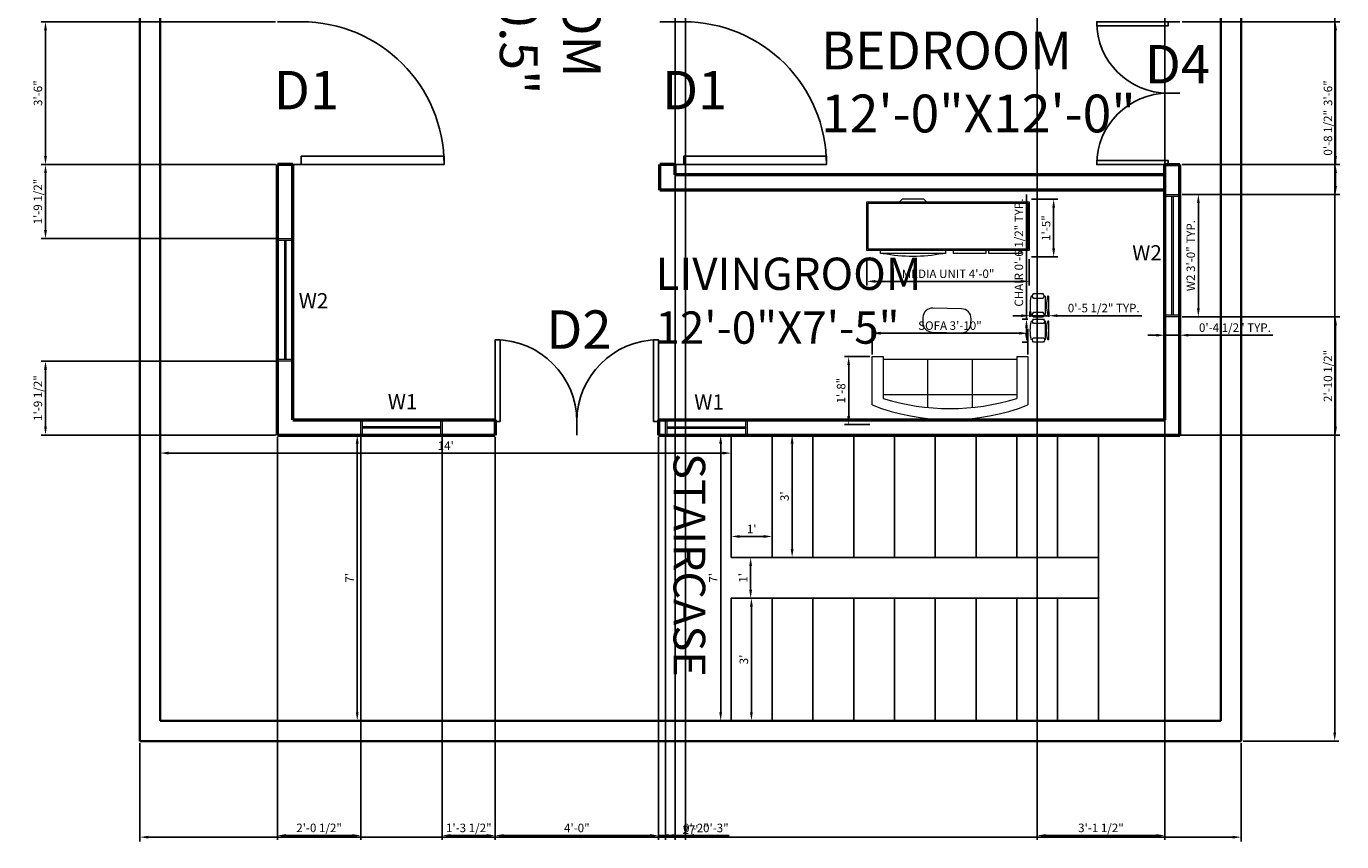
# Model space of a CAD drawing. Units: inches. Extents: x 2727 to 5054, y 1285 to 3233.
# Tile 1 of 3: x 2727 to 3114, y 1285 to 1525. Entities that reach past the tile are written whole.
import ezdxf

# ---------------------------------------------------------------- set-up
doc = ezdxf.new("R2010")
doc.units = ezdxf.units.IN
for name, color, linetype, lineweight in [('A-ANNO-TEXT', 1, 'Continuous', 18), ('A-AREA-IDEN', 1, 'Continuous', 18), ('A-WALL-SITE', 7, 'Continuous', 35), ('DIMENSIONS', 9, 'Continuous', 18), ('doors', 5, 'Continuous', 25), ('furniture', 8, 'Continuous', 18), ('stair case', 6, 'Continuous', 25), ('walls', 7, 'Continuous', 50), ('windows', 3, 'Continuous', 18)]:
    doc.layers.add(name, color=color, linetype=linetype, lineweight=lineweight)
doc.styles.get("Standard").update_dxf_attribs({"font": 'arial.ttf'})
doc.dimstyles.new('ISO-25', dxfattribs={"dimtxt": 2.5, "dimasz": 2.5, "dimexe": 1.25, "dimexo": 0.625, "dimtad": 1, "dimlunit": 4, "dimtxsty": 'Standard', "dimcen": 2.5, "dimadec": 0, "dimazin": 0, "dimtfac": 1, "dimtmove": 0, "dimatfit": 3, "dimfxl": 1, "dimarcsym": 0})

# ---------------------------------------------------------------- blocks, each defined once
blk = doc.blocks.new('*U2')
for p, q in [((0, 0), (0, -5)), ((30, 0), (30, -5))]:
    blk.add_line(p, q)
blk.add_lwpolyline([(0, 0), (0, 30), (1.75, 30), (1.75, 0)], close=True)
blk.add_arc((0, 0), 30, 0, 90)
blk = doc.blocks.new('Sofa - Roundback 7 ft.')
for p, q in [((-12.00002, -32.4421), (-12.00003, -6.5971)), ((11.99997, -32.4421), (11.99998, -6.5971)), ((-36.000027, -34), (-36.000027, -11.4696)), ((-35.999844, -13.3819), (35.9998, -13.3819)), ((35.99998, -34), (35.99998, -11.4696)), ((-36.000027, -32.4421), (35.99998, -32.4421))]:
    blk.add_line(p, q)
for points in [[(-36.000027, -34), (-42.000027, -34), (-42.000027, -8)], [(41.99998, -8), (41.99998, -34), (35.99998, -34)]]:
    blk.add_lwpolyline(points)
for centre, radius, start, end in [((0, -114.25), 114.25, 68.43141, 111.5686), ((-0.00001, -127.1968), 121.1968, 72.72033, 107.2797)]:
    blk.add_arc(centre, radius, start, end)
blk = doc.blocks.new('Chair - Desk')
for p, q in [((-8.5, 0), (-8.5, -1)), ((-8.5, 0), (8.5, 0)), ((8.5, 0), (8.5, -1)), ((-10.5, -5), (-10.5, -14)), ((-8.5, -3), (-8.5, -4)), ((-8.5, -3), (8.5, -3)), ((-6.5, -14), (-6.5, -5)), ((-2, -3), (-2, -1.9355)), ((2, -1.9576), (2, -3)), ((6.5, -5), (6.5, -14)), ((8.5, -3), (8.5, -4)), ((10.5, -14), (10.5, -5)), ((-8.5, -15), (-8.5, -16)), ((8.5, -15), (8.5, -16))]:
    blk.add_line(p, q)
for centre, radius, start, end in [((-8.5, -6.5), 2.5, 36.8699, 143.1301), ((0, 34.625), 36.625, 256.5803, 283.4197), ((8.5, -6.5), 2.5, 36.8699, 143.1301), ((-8.5, -12.5), 2.5, 216.8699, 323.1301), ((0, 19.625), 36.625, 256.5803, 283.4197), ((8.5, -12.5), 2.5, 216.8699, 323.1301)]:
    blk.add_arc(centre, radius, start, end)
blk = doc.blocks.new('Entertainment Center')
for p, q in [((-4, 0), (-5, -1)), ((4, 0), (-4, 0)), ((5, -1), (4, 0)), ((-17, -19), (-17, -1)), ((-17, -1), (43, -1)), ((-16.5, -18.5), (-16.5, -1.5)), ((-16.5, -1.5), (42.5, -1.5)), ((42.5, -1.5), (42.5, -18.5)), ((43, -1), (43, -19)), ((43, -19), (-17, -19)), ((42.5, -18.5), (-16.5, -18.5)), ((-12, -20), (-12, -19)), ((12, -19), (12, -20)), ((15, -20), (15, -19)), ((27, -19), (27, -20)), ((28, -20), (28, -19)), ((40, -19), (40, -20)), ((12, -20), (-12, -20)), ((27, -20), (15, -20)), ((40, -20), (28, -20))]:
    blk.add_line(p, q)
blk.add_arc((0, 40), 61, 259.6111, 280.3889)
blk = doc.blocks.new('*D9')
at = {"layer": 'Defpoints', "color": 0, "transparency": 16777216}
for p in [(3084.39, 1866.39), (3084.39, 1314.39), (3111.91, 1314.39)]:
    blk.add_point(p, dxfattribs=at)
at = {"layer": 'DIMENSIONS', "color": 0, "lineweight": -2, "transparency": 16777216}
for p, q in [((3085.02, 1866.39), (3113.16, 1866.39)), ((3111.91, 1863.89), (3111.91, 1316.89)), ((3085.02, 1314.39), (3113.16, 1314.39))]:
    blk.add_line(p, q, dxfattribs=at)
at = {"layer": 'DIMENSIONS', "color": 0, "transparency": 16777216}
for points in [[(3111.49, 1863.89), (3112.33, 1863.89), (3111.91, 1866.39)], [(3111.49, 1316.89), (3112.33, 1316.89), (3111.91, 1314.39)]]:
    blk.add_solid(points, dxfattribs=at)
at = {"layer": 'DIMENSIONS', "color": 0, "transparency": 16777216, "insert": (3110.01, 1590.39), "char_height": 2.5, "attachment_point": 5, "rotation": 90}
blk.add_mtext("46'", dxfattribs=at)
blk = doc.blocks.new('*D10')
at = {"layer": 'Defpoints', "color": 0, "transparency": 16777216}
for p in [(2760.39, 1314.39), (3084.39, 1314.39), (3084.39, 1286.15)]:
    blk.add_point(p, dxfattribs=at)
at = {"layer": 'DIMENSIONS', "color": 0, "lineweight": -2, "transparency": 16777216}
for p, q in [((2760.39, 1313.77), (2760.39, 1284.9)), ((3084.39, 1313.77), (3084.39, 1284.9)), ((2762.89, 1286.15), (3081.89, 1286.15))]:
    blk.add_line(p, q, dxfattribs=at)
at = {"layer": 'DIMENSIONS', "color": 0, "transparency": 16777216}
for points in [[(2762.89, 1286.56), (2762.89, 1285.73), (2760.39, 1286.15)], [(3081.89, 1286.56), (3081.89, 1285.73), (3084.39, 1286.15)]]:
    blk.add_solid(points, dxfattribs=at)
at = {"layer": 'DIMENSIONS', "color": 0, "transparency": 16777216, "insert": (2922.39, 1288.03), "char_height": 2.5, "attachment_point": 5}
blk.add_mtext("27'", dxfattribs=at)
blk = doc.blocks.new('*D16')
at = {"layer": 'Defpoints', "color": 0, "transparency": 16777216}
for p in [(2815.23, 1404.39), (2815.23, 1320.39), (2824.34, 1320.39)]:
    blk.add_point(p, dxfattribs=at)
at = {"layer": 'DIMENSIONS', "color": 0, "lineweight": -2, "transparency": 16777216}
for p, q in [((2815.85, 1404.39), (2825.59, 1404.39)), ((2824.34, 1401.89), (2824.34, 1322.89)), ((2815.85, 1320.39), (2825.59, 1320.39))]:
    blk.add_line(p, q, dxfattribs=at)
at = {"layer": 'DIMENSIONS', "color": 0, "transparency": 16777216}
for points in [[(2823.92, 1401.89), (2824.76, 1401.89), (2824.34, 1404.39)], [(2823.92, 1322.89), (2824.76, 1322.89), (2824.34, 1320.39)]]:
    blk.add_solid(points, dxfattribs=at)
at = {"layer": 'DIMENSIONS', "color": 0, "transparency": 16777216, "insert": (2822.46, 1362.39), "char_height": 2.5, "attachment_point": 5, "rotation": 90}
blk.add_mtext("7'", dxfattribs=at)
blk = doc.blocks.new('*D17')
at = {"layer": 'Defpoints', "color": 0, "transparency": 16777216}
for p in [(2934.39, 1399.07), (2766.39, 1382.65), (2934.39, 1382.65)]:
    blk.add_point(p, dxfattribs=at)
at = {"layer": 'DIMENSIONS', "color": 0, "lineweight": -2, "transparency": 16777216}
for p, q in [((2766.39, 1383.28), (2766.39, 1400.32)), ((2768.89, 1399.07), (2931.89, 1399.07)), ((2934.39, 1383.28), (2934.39, 1400.32))]:
    blk.add_line(p, q, dxfattribs=at)
at = {"layer": 'DIMENSIONS', "color": 0, "transparency": 16777216}
for points in [[(2768.89, 1399.49), (2768.89, 1398.66), (2766.39, 1399.07)], [(2931.89, 1399.49), (2931.89, 1398.66), (2934.39, 1399.07)]]:
    blk.add_solid(points, dxfattribs=at)
at = {"layer": 'DIMENSIONS', "color": 0, "transparency": 16777216, "insert": (2850.39, 1400.95), "char_height": 2.5, "attachment_point": 5}
blk.add_mtext("14'", dxfattribs=at)
blk = doc.blocks.new('*D18')
at = {"layer": 'Defpoints', "color": 0, "transparency": 16777216}
for p in [(2946.39, 1374.56), (2934.39, 1368.39), (2946.39, 1368.39)]:
    blk.add_point(p, dxfattribs=at)
at = {"layer": 'DIMENSIONS', "color": 0, "lineweight": -2, "transparency": 16777216}
for p, q in [((2934.39, 1369.02), (2934.39, 1375.81)), ((2936.89, 1374.56), (2943.89, 1374.56)), ((2946.39, 1369.02), (2946.39, 1375.81))]:
    blk.add_line(p, q, dxfattribs=at)
at = {"layer": 'DIMENSIONS', "color": 0, "transparency": 16777216}
for points in [[(2936.89, 1374.97), (2936.89, 1374.14), (2934.39, 1374.56)], [(2943.89, 1374.97), (2943.89, 1374.14), (2946.39, 1374.56)]]:
    blk.add_solid(points, dxfattribs=at)
at = {"layer": 'DIMENSIONS', "color": 0, "transparency": 16777216, "insert": (2940.39, 1376.44), "char_height": 2.5, "attachment_point": 5}
blk.add_mtext("1'", dxfattribs=at)
blk = doc.blocks.new('*D19')
at = {"layer": 'Defpoints', "color": 0, "transparency": 16777216}
for p in [(2946.39, 1404.39), (2946.39, 1368.39), (2952.28, 1368.39)]:
    blk.add_point(p, dxfattribs=at)
at = {"layer": 'DIMENSIONS', "color": 0, "lineweight": -2, "transparency": 16777216}
for p, q in [((2947.02, 1404.39), (2953.53, 1404.39)), ((2952.28, 1401.89), (2952.28, 1370.89)), ((2947.02, 1368.39), (2953.53, 1368.39))]:
    blk.add_line(p, q, dxfattribs=at)
at = {"layer": 'DIMENSIONS', "color": 0, "transparency": 16777216}
for points in [[(2951.86, 1401.89), (2952.7, 1401.89), (2952.28, 1404.39)], [(2951.86, 1370.89), (2952.7, 1370.89), (2952.28, 1368.39)]]:
    blk.add_solid(points, dxfattribs=at)
at = {"layer": 'DIMENSIONS', "color": 0, "transparency": 16777216, "insert": (2950.38, 1386.39), "char_height": 2.5, "attachment_point": 5, "rotation": 90}
blk.add_mtext("3'", dxfattribs=at)
blk = doc.blocks.new('*D20')
at = {"layer": 'Defpoints', "color": 0, "transparency": 16777216}
for p in [(2934.39, 1368.39), (2934.39, 1356.39), (2940.08, 1356.39)]:
    blk.add_point(p, dxfattribs=at)
at = {"layer": 'DIMENSIONS', "color": 0, "lineweight": -2, "transparency": 16777216}
for p, q in [((2935.02, 1368.39), (2941.33, 1368.39)), ((2940.08, 1365.89), (2940.08, 1358.89)), ((2935.02, 1356.39), (2941.33, 1356.39))]:
    blk.add_line(p, q, dxfattribs=at)
at = {"layer": 'DIMENSIONS', "color": 0, "transparency": 16777216}
for points in [[(2939.66, 1365.89), (2940.49, 1365.89), (2940.08, 1368.39)], [(2939.66, 1358.89), (2940.49, 1358.89), (2940.08, 1356.39)]]:
    blk.add_solid(points, dxfattribs=at)
at = {"layer": 'DIMENSIONS', "color": 0, "transparency": 16777216, "insert": (2938.2, 1362.39), "char_height": 2.5, "attachment_point": 5, "rotation": 90}
blk.add_mtext("1'", dxfattribs=at)
blk = doc.blocks.new('*D21')
at = {"layer": 'Defpoints', "color": 0, "transparency": 16777216}
for p in [(2934.39, 1356.39), (2940.31, 1356.39), (2934.39, 1320.39)]:
    blk.add_point(p, dxfattribs=at)
at = {"layer": 'DIMENSIONS', "color": 0, "lineweight": -2, "transparency": 16777216}
for p, q in [((2935.02, 1356.39), (2941.56, 1356.39)), ((2940.31, 1322.89), (2940.31, 1353.89)), ((2935.02, 1320.39), (2941.56, 1320.39))]:
    blk.add_line(p, q, dxfattribs=at)
at = {"layer": 'DIMENSIONS', "color": 0, "transparency": 16777216}
for points in [[(2939.89, 1353.89), (2940.72, 1353.89), (2940.31, 1356.39)], [(2939.89, 1322.89), (2940.72, 1322.89), (2940.31, 1320.39)]]:
    blk.add_solid(points, dxfattribs=at)
at = {"layer": 'DIMENSIONS', "color": 0, "transparency": 16777216, "insert": (2938.4, 1338.39), "char_height": 2.5, "attachment_point": 5, "rotation": 90}
blk.add_mtext("3'", dxfattribs=at)
blk = doc.blocks.new('*D22')
at = {"layer": 'Defpoints', "color": 0, "transparency": 16777216}
for p in [(2931.27, 1404.39), (2934.39, 1404.39), (2934.39, 1320.39)]:
    blk.add_point(p, dxfattribs=at)
at = {"layer": 'DIMENSIONS', "color": 0, "lineweight": -2, "transparency": 16777216}
for p, q in [((2933.77, 1404.39), (2930.02, 1404.39)), ((2931.27, 1322.89), (2931.27, 1401.89)), ((2933.77, 1320.39), (2930.02, 1320.39))]:
    blk.add_line(p, q, dxfattribs=at)
at = {"layer": 'DIMENSIONS', "color": 0, "transparency": 16777216}
for points in [[(2930.85, 1401.89), (2931.68, 1401.89), (2931.27, 1404.39)], [(2930.85, 1322.89), (2931.68, 1322.89), (2931.27, 1320.39)]]:
    blk.add_solid(points, dxfattribs=at)
at = {"layer": 'DIMENSIONS', "color": 0, "transparency": 16777216, "insert": (2929.39, 1362.39), "char_height": 2.5, "attachment_point": 5, "rotation": 90}
blk.add_mtext("7'", dxfattribs=at)
blk = doc.blocks.new('WIN-W1-24IN')
for p, q in [((0, 4.5), (24.02, 4.5)), ((0, 0), (0, 4.5)), ((0.5, 0), (0.5, 4.5)), ((23.52, 4.5), (23.52, 0)), ((24.02, 4.5), (24.02, 0)), ((24.02, 0), (0, 0)), ((0.5, 2.45), (23.52, 2.45)), ((0.5, 2.05), (23.52, 2.05))]:
    blk.add_line(p, q)
blk = doc.blocks.new('WIN-W2-36IN')
for p, q in [((0, 0), (0, 36.02)), ((0, 36.02), (4.5, 36.02)), ((0, 35.52), (4.5, 35.52)), ((2.05, 35.52), (2.05, 0.5)), ((2.45, 35.52), (2.45, 0.5)), ((4.5, 36.02), (4.5, 0)), ((4.5, 0.5), (0, 0.5)), ((4.5, 0), (0, 0))]:
    blk.add_line(p, q)
blk = doc.blocks.new('*D27')
at = {"layer": 'Defpoints', "color": 0, "transparency": 16777216}
for p in [(3066.39, 1475.14), (3071.79, 1475.14), (3066.39, 1439.13)]:
    blk.add_point(p, dxfattribs=at)
at = {"layer": 'DIMENSIONS', "color": 0, "lineweight": -2, "transparency": 16777216}
for p, q in [((3067.02, 1475.14), (3073.04, 1475.14)), ((3071.79, 1441.63), (3071.79, 1472.64)), ((3067.02, 1439.13), (3073.04, 1439.13))]:
    blk.add_line(p, q, dxfattribs=at)
at = {"layer": 'DIMENSIONS', "color": 0, "transparency": 16777216}
for points in [[(3071.38, 1472.64), (3072.21, 1472.64), (3071.79, 1475.14)], [(3071.38, 1441.63), (3072.21, 1441.63), (3071.79, 1439.13)]]:
    blk.add_solid(points, dxfattribs=at)
at = {"layer": 'DIMENSIONS', "color": 0, "transparency": 16777216, "insert": (3069.89, 1457.13), "char_height": 2.5, "attachment_point": 5, "rotation": 90}
blk.add_mtext('W2 3\'-0" TYP.', dxfattribs=at)
blk = doc.blocks.new('*D28')
at = {"layer": 'Defpoints', "color": 0, "transparency": 16777216}
for p in [(3061.89, 1439.13), (3066.39, 1439.13), (3066.39, 1433.72)]:
    blk.add_point(p, dxfattribs=at)
at = {"layer": 'DIMENSIONS', "color": 0, "lineweight": -2, "transparency": 16777216}
for p, q in [((3061.89, 1438.5), (3061.89, 1432.47)), ((3066.39, 1438.5), (3066.39, 1432.47)), ((3059.39, 1433.72), (3056.89, 1433.72)), ((3061.89, 1433.72), (3066.39, 1433.72)), ((3068.89, 1433.72), (3093.7, 1433.72))]:
    blk.add_line(p, q, dxfattribs=at)
at = {"layer": 'DIMENSIONS', "color": 0, "transparency": 16777216}
for points in [[(3059.39, 1434.14), (3059.39, 1433.31), (3061.89, 1433.72)], [(3068.89, 1434.14), (3068.89, 1433.31), (3066.39, 1433.72)]]:
    blk.add_solid(points, dxfattribs=at)
at = {"layer": 'DIMENSIONS', "color": 0, "transparency": 16777216, "insert": (3082.55, 1435.64), "char_height": 2.5, "attachment_point": 5}
blk.add_mtext('0\'-4 1/2" TYP.', dxfattribs=at)
blk = doc.blocks.new('*D29')
at = {"layer": 'Defpoints', "color": 0, "transparency": 16777216}
for p in [(3021.23, 1438.46), (3022.24, 1438.46), (3022.24, 1431.72)]:
    blk.add_point(p, dxfattribs=at)
at = {"layer": 'DIMENSIONS', "color": 0, "lineweight": -2, "transparency": 16777216}
for p, q in [((3021.23, 1438.46), (3021.23, 1475.08)), ((3021.62, 1438.46), (3019.98, 1438.46)), ((3021.23, 1434.22), (3021.23, 1435.96)), ((3021.62, 1431.72), (3019.98, 1431.72))]:
    blk.add_line(p, q, dxfattribs=at)
at = {"layer": 'DIMENSIONS', "color": 0, "transparency": 16777216}
for points in [[(3020.81, 1435.96), (3021.65, 1435.96), (3021.23, 1438.46)], [(3020.81, 1434.22), (3021.65, 1434.22), (3021.23, 1431.72)]]:
    blk.add_solid(points, dxfattribs=at)
at = {"layer": 'DIMENSIONS', "color": 0, "transparency": 16777216, "insert": (3019.31, 1458.02), "char_height": 2.5, "attachment_point": 5, "rotation": 90}
blk.add_mtext('CHAIR 0\'-6 1/2" TYP.', dxfattribs=at)
blk = doc.blocks.new('*D30')
at = {"layer": 'Defpoints', "color": 0, "transparency": 16777216}
for p in [(3022.24, 1438.46), (3027.81, 1439.47), (3027.81, 1438.46)]:
    blk.add_point(p, dxfattribs=at)
at = {"layer": 'DIMENSIONS', "color": 0, "lineweight": -2, "transparency": 16777216}
for p, q in [((3022.24, 1439.09), (3022.24, 1440.72)), ((3027.81, 1439.09), (3027.81, 1440.72)), ((3019.74, 1439.47), (3017.24, 1439.47)), ((3022.24, 1439.47), (3027.81, 1439.47)), ((3030.31, 1439.47), (3055.12, 1439.47))]:
    blk.add_line(p, q, dxfattribs=at)
at = {"layer": 'DIMENSIONS', "color": 0, "transparency": 16777216}
for points in [[(3019.74, 1439.89), (3019.74, 1439.05), (3022.24, 1439.47)], [(3030.31, 1439.89), (3030.31, 1439.05), (3027.81, 1439.47)]]:
    blk.add_solid(points, dxfattribs=at)
at = {"layer": 'DIMENSIONS', "color": 0, "transparency": 16777216, "insert": (3043.96, 1441.39), "char_height": 2.5, "attachment_point": 5}
blk.add_mtext('0\'-5 1/2" TYP.', dxfattribs=at)
blk = doc.blocks.new('*D35')
at = {"layer": 'Defpoints', "color": 0, "transparency": 16777216}
for p in [(2975.79, 1434.31), (2975.79, 1427.44), (3021.62, 1427.44)]:
    blk.add_point(p, dxfattribs=at)
at = {"layer": 'DIMENSIONS', "color": 0, "lineweight": -2, "transparency": 16777216}
for p, q in [((2975.79, 1428.06), (2975.79, 1435.56)), ((3019.12, 1434.31), (2978.29, 1434.31)), ((3021.62, 1428.06), (3021.62, 1435.56))]:
    blk.add_line(p, q, dxfattribs=at)
at = {"layer": 'DIMENSIONS', "color": 0, "transparency": 16777216}
for points in [[(2978.29, 1434.73), (2978.29, 1433.9), (2975.79, 1434.31)], [(3019.12, 1434.73), (3019.12, 1433.9), (3021.62, 1434.31)]]:
    blk.add_solid(points, dxfattribs=at)
at = {"layer": 'DIMENSIONS', "color": 0, "transparency": 16777216, "insert": (2998.7, 1436.23), "char_height": 2.5, "attachment_point": 5}
blk.add_mtext('SOFA 3\'-10"', dxfattribs=at)
blk = doc.blocks.new('*D36')
at = {"layer": 'Defpoints', "color": 0, "transparency": 16777216}
for p in [(2975.79, 1427.44), (2968.92, 1407.44), (2975.79, 1407.44)]:
    blk.add_point(p, dxfattribs=at)
at = {"layer": 'DIMENSIONS', "color": 0, "lineweight": -2, "transparency": 16777216}
for p, q in [((2975.17, 1427.44), (2967.67, 1427.44)), ((2968.92, 1424.94), (2968.92, 1409.94)), ((2975.17, 1407.44), (2967.67, 1407.44))]:
    blk.add_line(p, q, dxfattribs=at)
at = {"layer": 'DIMENSIONS', "color": 0, "transparency": 16777216}
for points in [[(2968.5, 1424.94), (2969.33, 1424.94), (2968.92, 1427.44)], [(2968.5, 1409.94), (2969.33, 1409.94), (2968.92, 1407.44)]]:
    blk.add_solid(points, dxfattribs=at)
at = {"layer": 'DIMENSIONS', "color": 0, "transparency": 16777216, "insert": (2967.02, 1417.44), "char_height": 2.5, "attachment_point": 5, "rotation": 90}
blk.add_mtext('1\'-8"', dxfattribs=at)
blk = doc.blocks.new('*D39')
at = {"layer": 'Defpoints', "color": 0, "transparency": 16777216}
for p in [(2974.28, 1456.74), (3022.06, 1456.74), (3022.06, 1449.57)]:
    blk.add_point(p, dxfattribs=at)
at = {"layer": 'DIMENSIONS', "color": 0, "lineweight": -2, "transparency": 16777216}
for p, q in [((2974.28, 1456.11), (2974.28, 1448.32)), ((3022.06, 1456.11), (3022.06, 1448.32)), ((2976.78, 1449.57), (3019.56, 1449.57))]:
    blk.add_line(p, q, dxfattribs=at)
at = {"layer": 'DIMENSIONS', "color": 0, "transparency": 16777216}
for points in [[(2976.78, 1449.99), (2976.78, 1449.15), (2974.28, 1449.57)], [(3019.56, 1449.99), (3019.56, 1449.15), (3022.06, 1449.57)]]:
    blk.add_solid(points, dxfattribs=at)
at = {"layer": 'DIMENSIONS', "color": 0, "transparency": 16777216, "insert": (2998.17, 1451.47), "char_height": 2.5, "attachment_point": 5}
blk.add_mtext('MEDIA UNIT 4\'-0"', dxfattribs=at)
blk = doc.blocks.new('*D40')
at = {"layer": 'Defpoints', "color": 0, "transparency": 16777216}
for p in [(3022.06, 1473.72), (3029.22, 1473.72), (3022.06, 1456.74)]:
    blk.add_point(p, dxfattribs=at)
at = {"layer": 'DIMENSIONS', "color": 0, "lineweight": -2, "transparency": 16777216}
for p, q in [((3022.68, 1473.72), (3030.47, 1473.72)), ((3029.22, 1459.24), (3029.22, 1471.22)), ((3022.68, 1456.74), (3030.47, 1456.74))]:
    blk.add_line(p, q, dxfattribs=at)
at = {"layer": 'DIMENSIONS', "color": 0, "transparency": 16777216}
for points in [[(3028.81, 1471.22), (3029.64, 1471.22), (3029.22, 1473.72)], [(3028.81, 1459.24), (3029.64, 1459.24), (3029.22, 1456.74)]]:
    blk.add_solid(points, dxfattribs=at)
at = {"layer": 'DIMENSIONS', "color": 0, "transparency": 16777216, "insert": (3027.32, 1465.23), "char_height": 2.5, "attachment_point": 5, "rotation": 90}
blk.add_mtext('1\'-5"', dxfattribs=at)
blk = doc.blocks.new('*D42')
at = {"layer": 'Defpoints', "color": 0, "transparency": 16777216}
for p in [(2732.63, 1483.89), (2800.89, 1483.89), (2800.89, 1462.15)]:
    blk.add_point(p, dxfattribs=at)
at = {"layer": 'DIMENSIONS', "color": 0, "lineweight": -2, "transparency": 16777216}
for p, q in [((2800.27, 1483.89), (2731.38, 1483.89)), ((2732.63, 1464.65), (2732.63, 1481.39)), ((2800.27, 1462.15), (2731.38, 1462.15))]:
    blk.add_line(p, q, dxfattribs=at)
at = {"layer": 'DIMENSIONS', "color": 0, "transparency": 16777216}
for points in [[(2732.21, 1481.39), (2733.05, 1481.39), (2732.63, 1483.89)], [(2732.21, 1464.65), (2733.05, 1464.65), (2732.63, 1462.15)]]:
    blk.add_solid(points, dxfattribs=at)
at = {"layer": 'DIMENSIONS', "color": 0, "transparency": 16777216, "insert": (2730.71, 1473.02), "char_height": 2.5, "attachment_point": 5, "rotation": 90}
blk.add_mtext('1\'-9 1/2"', dxfattribs=at)
blk = doc.blocks.new('*D43')
at = {"layer": 'Defpoints', "color": 0, "transparency": 16777216}
for p in [(2732.63, 1525.89), (2800.89, 1525.89), (2800.89, 1483.89)]:
    blk.add_point(p, dxfattribs=at)
at = {"layer": 'DIMENSIONS', "color": 0, "lineweight": -2, "transparency": 16777216}
for p, q in [((2800.27, 1525.89), (2731.38, 1525.89)), ((2732.63, 1486.39), (2732.63, 1523.39)), ((2800.27, 1483.89), (2731.38, 1483.89))]:
    blk.add_line(p, q, dxfattribs=at)
at = {"layer": 'DIMENSIONS', "color": 0, "transparency": 16777216}
for points in [[(2732.21, 1523.39), (2733.05, 1523.39), (2732.63, 1525.89)], [(2732.21, 1486.39), (2733.05, 1486.39), (2732.63, 1483.89)]]:
    blk.add_solid(points, dxfattribs=at)
at = {"layer": 'DIMENSIONS', "color": 0, "transparency": 16777216, "insert": (2730.73, 1504.89), "char_height": 2.5, "attachment_point": 5, "rotation": 90}
blk.add_mtext('3\'-6"', dxfattribs=at)
blk = doc.blocks.new('*D44')
at = {"layer": 'Defpoints', "color": 0, "transparency": 16777216}
for p in [(2864.94, 1404.39), (2912.94, 1404.39), (2912.94, 1286.63)]:
    blk.add_point(p, dxfattribs=at)
at = {"layer": 'DIMENSIONS', "color": 0, "lineweight": -2, "transparency": 16777216}
for p, q in [((2864.94, 1403.77), (2864.94, 1285.38)), ((2912.94, 1403.77), (2912.94, 1285.38)), ((2867.44, 1286.63), (2910.44, 1286.63))]:
    blk.add_line(p, q, dxfattribs=at)
at = {"layer": 'DIMENSIONS', "color": 0, "transparency": 16777216}
for points in [[(2867.44, 1287.05), (2867.44, 1286.21), (2864.94, 1286.63)], [(2910.44, 1287.05), (2910.44, 1286.21), (2912.94, 1286.63)]]:
    blk.add_solid(points, dxfattribs=at)
at = {"layer": 'DIMENSIONS', "color": 0, "transparency": 16777216, "insert": (2888.94, 1288.53), "char_height": 2.5, "attachment_point": 5}
blk.add_mtext('4\'-0"', dxfattribs=at)
blk = doc.blocks.new('*D47')
at = {"layer": 'Defpoints', "color": 0, "transparency": 16777216}
for p in [(2849.37, 1404.39), (2864.94, 1404.39), (2864.94, 1286.63)]:
    blk.add_point(p, dxfattribs=at)
at = {"layer": 'DIMENSIONS', "color": 0, "lineweight": -2, "transparency": 16777216}
for p, q in [((2849.37, 1403.77), (2849.37, 1285.38)), ((2864.94, 1403.77), (2864.94, 1285.38)), ((2851.87, 1286.63), (2862.44, 1286.63))]:
    blk.add_line(p, q, dxfattribs=at)
at = {"layer": 'DIMENSIONS', "color": 0, "transparency": 16777216}
for points in [[(2851.87, 1287.05), (2851.87, 1286.21), (2849.37, 1286.63)], [(2862.44, 1287.05), (2862.44, 1286.21), (2864.94, 1286.63)]]:
    blk.add_solid(points, dxfattribs=at)
at = {"layer": 'DIMENSIONS', "color": 0, "transparency": 16777216, "insert": (2857.16, 1288.55), "char_height": 2.5, "attachment_point": 5}
blk.add_mtext('1\'-3 1/2"', dxfattribs=at)
blk = doc.blocks.new('*D50')
at = {"layer": 'Defpoints', "color": 0, "transparency": 16777216}
for p in [(2732.63, 1426.13), (2800.89, 1426.13), (2800.89, 1404.39)]:
    blk.add_point(p, dxfattribs=at)
at = {"layer": 'DIMENSIONS', "color": 0, "lineweight": -2, "transparency": 16777216}
for p, q in [((2800.27, 1426.13), (2731.38, 1426.13)), ((2732.63, 1406.89), (2732.63, 1423.63)), ((2800.27, 1404.39), (2731.38, 1404.39))]:
    blk.add_line(p, q, dxfattribs=at)
at = {"layer": 'DIMENSIONS', "color": 0, "transparency": 16777216}
for points in [[(2732.21, 1423.63), (2733.05, 1423.63), (2732.63, 1426.13)], [(2732.21, 1406.89), (2733.05, 1406.89), (2732.63, 1404.39)]]:
    blk.add_solid(points, dxfattribs=at)
at = {"layer": 'DIMENSIONS', "color": 0, "transparency": 16777216, "insert": (2730.71, 1415.26), "char_height": 2.5, "attachment_point": 5, "rotation": 90}
blk.add_mtext('1\'-9 1/2"', dxfattribs=at)
blk = doc.blocks.new('*D51')
at = {"layer": 'Defpoints', "color": 0, "transparency": 16777216}
for p in [(3066.39, 1439.13), (3112.15, 1439.13), (3066.39, 1404.39)]:
    blk.add_point(p, dxfattribs=at)
at = {"layer": 'DIMENSIONS', "color": 0, "lineweight": -2, "transparency": 16777216}
for p, q in [((3067.02, 1439.13), (3113.4, 1439.13)), ((3112.15, 1406.89), (3112.15, 1436.63)), ((3067.02, 1404.39), (3113.4, 1404.39))]:
    blk.add_line(p, q, dxfattribs=at)
at = {"layer": 'DIMENSIONS', "color": 0, "transparency": 16777216}
for points in [[(3111.73, 1436.63), (3112.57, 1436.63), (3112.15, 1439.13)], [(3111.73, 1406.89), (3112.57, 1406.89), (3112.15, 1404.39)]]:
    blk.add_solid(points, dxfattribs=at)
at = {"layer": 'DIMENSIONS', "color": 0, "transparency": 16777216, "insert": (3110.23, 1421.76), "char_height": 2.5, "attachment_point": 5, "rotation": 90}
blk.add_mtext('2\'-10 1/2"', dxfattribs=at)
blk = doc.blocks.new('*D52')
at = {"layer": 'Defpoints', "color": 0, "transparency": 16777216}
for p in [(2800.89, 1404.39), (2825.36, 1404.39), (2825.36, 1286.63)]:
    blk.add_point(p, dxfattribs=at)
at = {"layer": 'DIMENSIONS', "color": 0, "lineweight": -2, "transparency": 16777216}
for p, q in [((2800.89, 1403.77), (2800.89, 1285.38)), ((2825.36, 1403.77), (2825.36, 1285.38)), ((2803.39, 1286.63), (2822.86, 1286.63))]:
    blk.add_line(p, q, dxfattribs=at)
at = {"layer": 'DIMENSIONS', "color": 0, "transparency": 16777216}
for points in [[(2803.39, 1287.05), (2803.39, 1286.21), (2800.89, 1286.63)], [(2822.86, 1287.05), (2822.86, 1286.21), (2825.36, 1286.63)]]:
    blk.add_solid(points, dxfattribs=at)
at = {"layer": 'DIMENSIONS', "color": 0, "transparency": 16777216, "insert": (2813.12, 1288.55), "char_height": 2.5, "attachment_point": 5}
blk.add_mtext('2\'-0 1/2"', dxfattribs=at)
blk = doc.blocks.new('*D53')
at = {"layer": 'Defpoints', "color": 0, "transparency": 16777216}
for p in [(2912.94, 1404.39), (2915.03, 1404.39), (2915.03, 1286.63)]:
    blk.add_point(p, dxfattribs=at)
at = {"layer": 'DIMENSIONS', "color": 0, "lineweight": -2, "transparency": 16777216}
for p, q in [((2912.94, 1403.77), (2912.94, 1285.38)), ((2915.03, 1403.77), (2915.03, 1285.38)), ((2910.44, 1286.63), (2907.94, 1286.63)), ((2912.94, 1286.63), (2915.03, 1286.63)), ((2917.53, 1286.63), (2927.93, 1286.63))]:
    blk.add_line(p, q, dxfattribs=at)
at = {"layer": 'DIMENSIONS', "color": 0, "transparency": 16777216}
for points in [[(2910.44, 1287.05), (2910.44, 1286.21), (2912.94, 1286.63)], [(2917.53, 1287.05), (2917.53, 1286.21), (2915.03, 1286.63)]]:
    blk.add_solid(points, dxfattribs=at)
at = {"layer": 'DIMENSIONS', "color": 0, "transparency": 16777216, "insert": (2923.98, 1288.53), "char_height": 2.5, "attachment_point": 5}
blk.add_mtext('0\'-2"', dxfattribs=at)
blk = doc.blocks.new('*D57')
at = {"layer": 'Defpoints', "color": 0, "transparency": 16777216}
for p in [(3066.39, 1525.89), (3112.15, 1525.89), (3066.39, 1483.89)]:
    blk.add_point(p, dxfattribs=at)
at = {"layer": 'DIMENSIONS', "color": 0, "lineweight": -2, "transparency": 16777216}
for p, q in [((3067.02, 1525.89), (3113.4, 1525.89)), ((3112.15, 1486.39), (3112.15, 1523.39)), ((3067.02, 1483.89), (3113.4, 1483.89))]:
    blk.add_line(p, q, dxfattribs=at)
at = {"layer": 'DIMENSIONS', "color": 0, "transparency": 16777216}
for points in [[(3111.73, 1523.39), (3112.57, 1523.39), (3112.15, 1525.89)], [(3111.73, 1486.39), (3112.57, 1486.39), (3112.15, 1483.89)]]:
    blk.add_solid(points, dxfattribs=at)
at = {"layer": 'DIMENSIONS', "color": 0, "transparency": 16777216, "insert": (3110.25, 1504.89), "char_height": 2.5, "attachment_point": 5, "rotation": 90}
blk.add_mtext('3\'-6"', dxfattribs=at)
blk = doc.blocks.new('*D61')
at = {"layer": 'Defpoints', "color": 0, "transparency": 16777216}
for p in [(3066.39, 1483.89), (3112.15, 1483.89), (3066.39, 1475.14)]:
    blk.add_point(p, dxfattribs=at)
at = {"layer": 'DIMENSIONS', "color": 0, "lineweight": -2, "transparency": 16777216}
for p, q in [((3112.15, 1483.89), (3112.15, 1500.11)), ((3067.02, 1483.89), (3113.4, 1483.89)), ((3112.15, 1477.64), (3112.15, 1481.39)), ((3067.02, 1475.14), (3113.4, 1475.14))]:
    blk.add_line(p, q, dxfattribs=at)
at = {"layer": 'DIMENSIONS', "color": 0, "transparency": 16777216}
for points in [[(3111.73, 1481.39), (3112.57, 1481.39), (3112.15, 1483.89)], [(3111.73, 1477.64), (3112.57, 1477.64), (3112.15, 1475.14)]]:
    blk.add_solid(points, dxfattribs=at)
at = {"layer": 'DIMENSIONS', "color": 0, "transparency": 16777216, "insert": (3110.23, 1493.25), "char_height": 2.5, "attachment_point": 5, "rotation": 90}
blk.add_mtext('0\'-8 1/2"', dxfattribs=at)
blk = doc.blocks.new('*D62')
at = {"layer": 'Defpoints', "color": 0, "transparency": 16777216}
for p in [(3024.39, 1675.89), (3061.89, 1675.89), (3061.89, 1286.63)]:
    blk.add_point(p, dxfattribs=at)
at = {"layer": 'DIMENSIONS', "color": 0, "lineweight": -2, "transparency": 16777216}
for p, q in [((3024.39, 1675.27), (3024.39, 1285.38)), ((3061.89, 1675.27), (3061.89, 1285.38)), ((3026.89, 1286.63), (3059.39, 1286.63))]:
    blk.add_line(p, q, dxfattribs=at)
at = {"layer": 'DIMENSIONS', "color": 0, "transparency": 16777216}
for points in [[(3026.89, 1287.05), (3026.89, 1286.21), (3024.39, 1286.63)], [(3059.39, 1287.05), (3059.39, 1286.21), (3061.89, 1286.63)]]:
    blk.add_solid(points, dxfattribs=at)
at = {"layer": 'DIMENSIONS', "color": 0, "transparency": 16777216, "insert": (3043.14, 1288.55), "char_height": 2.5, "attachment_point": 5}
blk.add_mtext('3\'-1 1/2"', dxfattribs=at)
blk = doc.blocks.new('*D63')
at = {"layer": 'Defpoints', "color": 0, "transparency": 16777216}
for p in [(2917.89, 1624.89), (2920.89, 1624.89), (2920.89, 1286.63)]:
    blk.add_point(p, dxfattribs=at)
at = {"layer": 'DIMENSIONS', "color": 0, "lineweight": -2, "transparency": 16777216}
for p, q in [((2917.89, 1624.27), (2917.89, 1285.38)), ((2920.89, 1624.27), (2920.89, 1285.38)), ((2915.39, 1286.63), (2912.89, 1286.63)), ((2917.89, 1286.63), (2920.89, 1286.63)), ((2923.39, 1286.63), (2933.79, 1286.63))]:
    blk.add_line(p, q, dxfattribs=at)
at = {"layer": 'DIMENSIONS', "color": 0, "transparency": 16777216}
for points in [[(2915.39, 1287.05), (2915.39, 1286.21), (2917.89, 1286.63)], [(2923.39, 1287.05), (2923.39, 1286.21), (2920.89, 1286.63)]]:
    blk.add_solid(points, dxfattribs=at)
at = {"layer": 'DIMENSIONS', "color": 0, "transparency": 16777216, "insert": (2929.84, 1288.53), "char_height": 2.5, "attachment_point": 5}
blk.add_mtext('0\'-3"', dxfattribs=at)

msp = doc.modelspace()

# ---------------------------------------------------------------- linework, layer by layer
at = {"layer": 'A-WALL-SITE'}
for p, q in [((2760.39, 1866.39), (2760.39, 1314.39)), ((3084.39, 1314.39), (3084.39, 1866.39)), ((2766.39, 1860.39), (2766.39, 1320.39)), ((3078.39, 1320.39), (3078.39, 1860.39)), ((2766.39, 1320.39), (3078.39, 1320.39)), ((2760.39, 1314.39), (3084.39, 1314.39))]:
    msp.add_line(p, q, dxfattribs=at)
at = {"layer": 'furniture'}
msp.add_lwpolyline([(2993.656, 1441.705, 0.4142136), (2990.755, 1438.946), (2990.719, 1437.53, 0.4142136), (2993.479, 1434.629), (3001.97, 1434.416, 0.4142136), (3004.871, 1437.175), (3004.907, 1438.591, 0.4142136), (3002.147, 1441.492)], format="xyb", close=True, dxfattribs=at)
at = {"layer": 'stair case'}
for p, q in [((3078.39, 1404.39), (2934.39, 1404.39)), ((2934.39, 1404.39), (2934.39, 1368.39)), ((2934.39, 1368.39), (2934.39, 1404.39)), ((2946.39, 1368.39), (2946.39, 1404.39)), ((2958.39, 1368.39), (2958.39, 1404.39)), ((2970.39, 1368.39), (2970.39, 1404.39)), ((2982.39, 1368.39), (2982.39, 1404.39)), ((2994.39, 1368.39), (2994.39, 1404.39)), ((3006.39, 1368.39), (3006.39, 1404.39)), ((3018.39, 1368.39), (3018.39, 1404.39)), ((3030.39, 1368.39), (3030.39, 1404.39)), ((3042.39, 1320.39), (3042.39, 1404.39)), ((3078.39, 1320.39), (3078.39, 1404.39)), ((3042.39, 1368.39), (2934.39, 1368.39)), ((2934.39, 1356.39), (3042.39, 1356.39)), ((2934.39, 1320.39), (2934.39, 1356.39)), ((2934.39, 1356.39), (2934.39, 1320.39)), ((2946.39, 1320.39), (2946.39, 1356.39)), ((2958.39, 1320.39), (2958.39, 1356.39)), ((2970.39, 1320.39), (2970.39, 1356.39)), ((2982.39, 1320.39), (2982.39, 1356.39)), ((2994.39, 1320.39), (2994.39, 1356.39)), ((3006.39, 1320.39), (3006.39, 1356.39)), ((3018.39, 1320.39), (3018.39, 1356.39)), ((3030.39, 1320.39), (3030.39, 1356.39)), ((2934.39, 1320.39), (3078.39, 1320.39))]:
    msp.add_line(p, q, dxfattribs=at)
at = {"layer": 'walls'}
for p, q in [((2800.89, 1404.39), (2800.89, 1483.89)), ((2805.39, 1483.89), (2800.89, 1483.89)), ((2805.39, 1408.89), (2805.39, 1483.89)), ((2913.39, 1476.39), (2913.39, 1483.89)), ((2917.89, 1483.89), (2913.39, 1483.89)), ((2917.89, 1480.89), (2917.89, 1483.89)), ((2917.89, 1480.89), (2917.89, 1483.89)), ((3061.89, 1408.89), (3061.89, 1483.89)), ((3061.89, 1483.89), (3066.39, 1483.89)), ((3066.39, 1404.39), (3066.39, 1483.89)), ((3061.89, 1480.89), (2917.89, 1480.89)), ((2917.89, 1480.89), (2917.89, 1480.89)), ((3061.89, 1476.39), (2913.39, 1476.39)), ((2805.39, 1408.89), (2864.944, 1408.89)), ((2864.944, 1408.89), (2864.944, 1404.39)), ((2912.944, 1408.89), (2912.944, 1404.39)), ((2912.944, 1408.89), (3061.89, 1408.89)), ((2800.89, 1404.39), (2864.944, 1404.39)), ((2912.944, 1404.39), (3066.39, 1404.39))]:
    msp.add_line(p, q, dxfattribs=at)

# ---------------------------------------------------------------- block references
at = {"layer": 'doors'}
for p, xscale, yscale, zscale, rotation in [((2807.89, 1483.89), -1.399999999999999, 1.399999999999999, 1.399999999999999, 270), ((2920.39, 1483.89), -1.399999999999999, 1.399999999999999, 1.399999999999999, 270), ((3062.89, 1525.89), -0.7, 0.7, 0.7, 90), ((3062.89, 1483.89), 0.7, 0.7, 0.7, 90.00000000000003)]:
    msp.add_blockref('*U2', p, dxfattribs=dict(at, xscale=xscale, yscale=yscale, zscale=zscale, rotation=rotation))
at = {"layer": 'doors', "yscale": 0.8, "zscale": 0.8}
for p, xscale in [((2864.944, 1408.39), 0.8), ((2912.944, 1408.39), -0.8)]:
    msp.add_blockref('*U2', p, dxfattribs=dict(at, xscale=xscale))
at = {"layer": 'furniture', "xscale": 0.7962554613330064, "yscale": 0.7962554613330064, "zscale": 0.7962554613330064}
msp.add_blockref('Entertainment Center', (2987.818, 1473.724), dxfattribs=at)
at = {"layer": 'furniture'}
for name, p, xscale, yscale, zscale, rotation in [('Chair - Desk', (3027.729, 1442.512), 0.3209796709069931, 0.3209796709069931, 0.3209796709069931, 270), ('Chair - Desk', (3027.805, 1435.09), -0.3209796709069931, 0.3209796709069931, 0.3209796709069931, 270), ('Sofa - Roundback 7 ft.', (2998.704, 1408.89), 0.5455526123410709, 0.5455526123410709, 0.5455526123410709, 180)]:
    msp.add_blockref(name, p, dxfattribs=dict(at, xscale=xscale, yscale=yscale, zscale=zscale, rotation=rotation))
at = {"layer": 'windows'}
for name, p in [('WIN-W2-36IN', (3061.89, 1439.126)), ('WIN-W2-36IN', (2800.89, 1426.133)), ('WIN-W1-24IN', (2915.03, 1404.39))]:
    msp.add_blockref(name, p, dxfattribs=at)
at = {"layer": 'windows', "rotation": 180}
msp.add_blockref('WIN-W1-24IN', (2849.373, 1408.89), dxfattribs=at)

# ---------------------------------------------------------------- texts
at = {"layer": 'A-ANNO-TEXT', "char_height": 11.3069, "attachment_point": 1}
for s, insert in [('D4', (3056.028, 1519.051)), ('D1', (2799.804, 1511.439)), ('D1', (2914.012, 1511.439)), ('D2', (2879.958, 1441.034))]:
    msp.add_mtext(s, dxfattribs=dict(at, insert=insert))
at = {"layer": 'A-ANNO-TEXT', "char_height": 4.4548, "attachment_point": 1}
for s, insert in [('W2', (3052.331, 1460.199)), ('W2', (2807.131, 1446.099)), ('W1', (2833.329, 1416.422)), ('W1', (2923.49, 1416.308))]:
    msp.add_mtext_dynamic_manual_height_columns(s, width=0.75599, gutter_width=22.274, heights=[0], dxfattribs=dict(at, insert=insert))
at = {"layer": 'A-AREA-IDEN', "attachment_point": 1, "rotation": 270}
for s, width, gutter_width, insert, char_height in [('LIVINGROOM\\P9\'-0"X22\'-0.5"', 20.03048, 55.595, (2895.951, 1601.252), 11.11906), ('STAIRCASE', 27.93529, 46.697, (2926.728, 1399.073), 9.3393)]:
    msp.add_mtext_dynamic_manual_height_columns(s, width=width, gutter_width=gutter_width, heights=[0], dxfattribs=dict(at, insert=insert, char_height=char_height))
at = {"layer": 'A-AREA-IDEN', "attachment_point": 1}
for s, width, gutter_width, insert, char_height in [('BEDROOM\\P12\'-0"X12\'-0"', 20.03048, 55.595, (2960.816, 1523.013), 11.11906), ('LIVINGROOM\\P12\'-0"X7\'-5"', 17.09851, 47.458, (2912.072, 1456.538), 9.4915)]:
    msp.add_mtext_dynamic_manual_height_columns(s, width=width, gutter_width=gutter_width, heights=[0], dxfattribs=dict(at, insert=insert, char_height=char_height))

# ---------------------------------------------------------------- dimensions: what is measured, and where the dimension line sits
at = {"layer": 'DIMENSIONS'}
for base, p1, p2, angle, override, picture, middle in [((3111.911, 1314.39), (3084.39, 1866.39), (3084.39, 1314.39), 90, {"dimclrd": 0, "dimclre": 0, "dimclrt": 0}, '*D9', (3110.01, 1590.39)), ((2732.63, 1525.89), (2800.89, 1483.89), (2800.89, 1525.89), 90, {"dimdec": 1, "dimlfac": 1, "dimrnd": 0, "dimzin": 1, "dimdsep": 46, "dimlunit": 4, "dimfrac": 2}, '*D43', (2730.728, 1504.89)), ((3112.15, 1525.89), (3066.39, 1483.89), (3066.39, 1525.89), 90, {"dimdec": 1, "dimlfac": 1, "dimrnd": 0, "dimzin": 1, "dimdsep": 46, "dimlunit": 4, "dimfrac": 2}, '*D57', (3110.248, 1504.89)), ((3112.15, 1483.89), (3066.39, 1475.142), (3066.39, 1483.89), 90, {"dimdec": 1, "dimlfac": 1, "dimrnd": 0, "dimzin": 1, "dimdsep": 46, "dimlunit": 4, "dimfrac": 2}, '*D61', (3110.233, 1493.251)), ((2732.63, 1483.89), (2800.89, 1462.148), (2800.89, 1483.89), 90, {"dimdec": 1, "dimlfac": 1, "dimrnd": 0, "dimzin": 1, "dimdsep": 46, "dimlunit": 4, "dimfrac": 2}, '*D42', (2730.713, 1473.019)), ((3029.223, 1473.724), (3022.057, 1456.737), (3022.057, 1473.724), 90, {"dimdec": 1, "dimlfac": 1, "dimrnd": 0, "dimzin": 1, "dimdsep": 46, "dimlunit": 4, "dimfrac": 2}, '*D40', (3027.322, 1465.231)), ((3112.15, 1439.126), (3066.39, 1404.39), (3066.39, 1439.126), 90, {"dimdec": 1, "dimlfac": 1, "dimrnd": 0, "dimzin": 1, "dimdsep": 46, "dimlunit": 4, "dimfrac": 2}, '*D51', (3110.233, 1421.758)), ((2732.63, 1426.132), (2800.89, 1404.39), (2800.89, 1426.132), 90, {"dimdec": 1, "dimlfac": 1, "dimrnd": 0, "dimzin": 1, "dimdsep": 46, "dimlunit": 4, "dimfrac": 2}, '*D50', (2730.713, 1415.261)), ((2968.917, 1407.435), (2975.791, 1427.439), (2975.791, 1407.435), 270, {"dimdec": 1, "dimlfac": 1, "dimrnd": 0, "dimzin": 1, "dimdsep": 46, "dimlunit": 4, "dimfrac": 2}, '*D36', (2967.015, 1417.437)), ((2824.34, 1320.39), (2815.226, 1404.39), (2815.226, 1320.39), 90, {"dimclrd": 0, "dimclre": 0, "dimclrt": 0}, '*D16', (2822.465, 1362.39)), ((2931.266, 1404.39), (2934.39, 1320.39), (2934.39, 1404.39), 90, {"dimclrd": 0, "dimclre": 0, "dimclrt": 0}, '*D22', (2929.391, 1362.39)), ((2952.279, 1368.39), (2946.39, 1404.39), (2946.39, 1368.39), 90, {"dimclrd": 0, "dimclre": 0, "dimclrt": 0}, '*D19', (2950.377, 1386.39)), ((2940.076, 1356.39), (2934.39, 1368.39), (2934.39, 1356.39), 90, {"dimclrd": 0, "dimclre": 0, "dimclrt": 0}, '*D20', (2938.196, 1362.39)), ((2940.307, 1356.39), (2934.39, 1320.39), (2934.39, 1356.39), 90, {"dimclrd": 0, "dimclre": 0, "dimclrt": 0}, '*D21', (2938.405, 1338.39))]:
    dim = msp.add_linear_dim(base=base, p1=p1, p2=p2, angle=angle, dimstyle='ISO-25', override=override, dxfattribs=at)
    dim.commit()
    dim.dimension.update_dxf_attribs({"geometry": picture, "text_midpoint": middle})
for base, p1, p2, override, picture, middle in [((3061.89, 1286.63), (3024.39, 1675.89), (3061.89, 1675.89), {"dimdec": 1, "dimlfac": 1, "dimrnd": 0, "dimzin": 1, "dimdsep": 46, "dimlunit": 4, "dimfrac": 2}, '*D62', (3043.14, 1288.549)), ((2920.89, 1286.63), (2917.89, 1624.89), (2920.89, 1624.89), {"dimdec": 1, "dimlfac": 1, "dimrnd": 0, "dimzin": 1, "dimdsep": 46, "dimlunit": 4, "dimfrac": 2}, '*D63', (2929.838, 1288.532)), ((2934.39, 1399.073), (2766.39, 1382.652), (2934.39, 1382.652), {"dimclrd": 0, "dimclre": 0, "dimclrt": 0}, '*D17', (2850.39, 1400.953)), ((2825.357, 1286.63), (2800.89, 1404.39), (2825.357, 1404.39), {"dimdec": 1, "dimlfac": 1, "dimrnd": 0, "dimzin": 1, "dimdsep": 46, "dimlunit": 4, "dimfrac": 2}, '*D52', (2813.124, 1288.548)), ((2864.944, 1286.63), (2849.373, 1404.39), (2864.944, 1404.39), {"dimdec": 1, "dimlfac": 1, "dimrnd": 0, "dimzin": 1, "dimdsep": 46, "dimlunit": 4, "dimfrac": 2}, '*D47', (2857.159, 1288.549)), ((2912.944, 1286.63), (2864.944, 1404.39), (2912.944, 1404.39), {"dimdec": 1, "dimlfac": 1, "dimrnd": 0, "dimzin": 1, "dimdsep": 46, "dimlunit": 4, "dimfrac": 2}, '*D44', (2888.944, 1288.532)), ((2915.03, 1286.63), (2912.944, 1404.39), (2915.03, 1404.39), {"dimdec": 1, "dimlfac": 1, "dimrnd": 0, "dimzin": 1, "dimdsep": 46, "dimlunit": 4, "dimfrac": 2}, '*D53', (2923.977, 1288.532)), ((2946.39, 1374.555), (2934.39, 1368.39), (2946.39, 1368.39), {"dimclrd": 0, "dimclre": 0, "dimclrt": 0}, '*D18', (2940.39, 1376.435)), ((3084.39, 1286.145), (2760.39, 1314.39), (3084.39, 1314.39), {"dimclrd": 0, "dimclre": 0, "dimclrt": 0}, '*D10', (2922.39, 1288.025))]:
    dim = msp.add_linear_dim(base=base, p1=p1, p2=p2, dimstyle='ISO-25', override=override, dxfattribs=at)
    dim.commit()
    dim.dimension.update_dxf_attribs({"geometry": picture, "text_midpoint": middle})
for base, p1, p2, angle, text, picture, middle in [((3021.23, 1438.46), (3022.241, 1431.72), (3022.241, 1438.46), 90, 'CHAIR <> TYP.', '*D29', (3019.313, 1458.021)), ((3071.793, 1475.142), (3066.39, 1439.126), (3066.39, 1475.142), 90, 'W2 <> TYP.', '*D27', (3069.891, 1457.134)), ((2975.791, 1434.313), (3021.617, 1427.439), (2975.791, 1427.439), 180, 'SOFA <>', '*D35', (2998.704, 1436.232))]:
    dim = msp.add_linear_dim(base=base, p1=p1, p2=p2, angle=angle, text=text, dimstyle='ISO-25', override={"dimdec": 1, "dimlfac": 1, "dimrnd": 0, "dimzin": 1, "dimdsep": 46, "dimlunit": 4, "dimfrac": 2}, dxfattribs=at)
    dim.commit()
    dim.dimension.update_dxf_attribs({"geometry": picture, "text_midpoint": middle})
for base, p1, p2, text, picture, middle in [((3022.057, 1449.571), (2974.282, 1456.737), (3022.057, 1456.737), 'MEDIA UNIT <>', '*D39', (2998.169, 1451.472)), ((3027.805, 1439.472), (3022.241, 1438.46), (3027.805, 1438.46), '<> TYP.', '*D30', (3043.962, 1441.389)), ((3066.39, 1433.723), (3061.89, 1439.126), (3066.39, 1439.126), '<> TYP.', '*D28', (3082.548, 1435.641))]:
    dim = msp.add_linear_dim(base=base, p1=p1, p2=p2, text=text, dimstyle='ISO-25', override={"dimdec": 1, "dimlfac": 1, "dimrnd": 0, "dimzin": 1, "dimdsep": 46, "dimlunit": 4, "dimfrac": 2}, dxfattribs=at)
    dim.commit()
    dim.dimension.update_dxf_attribs({"geometry": picture, "text_midpoint": middle})

doc.saveas('drawing.dxf')
